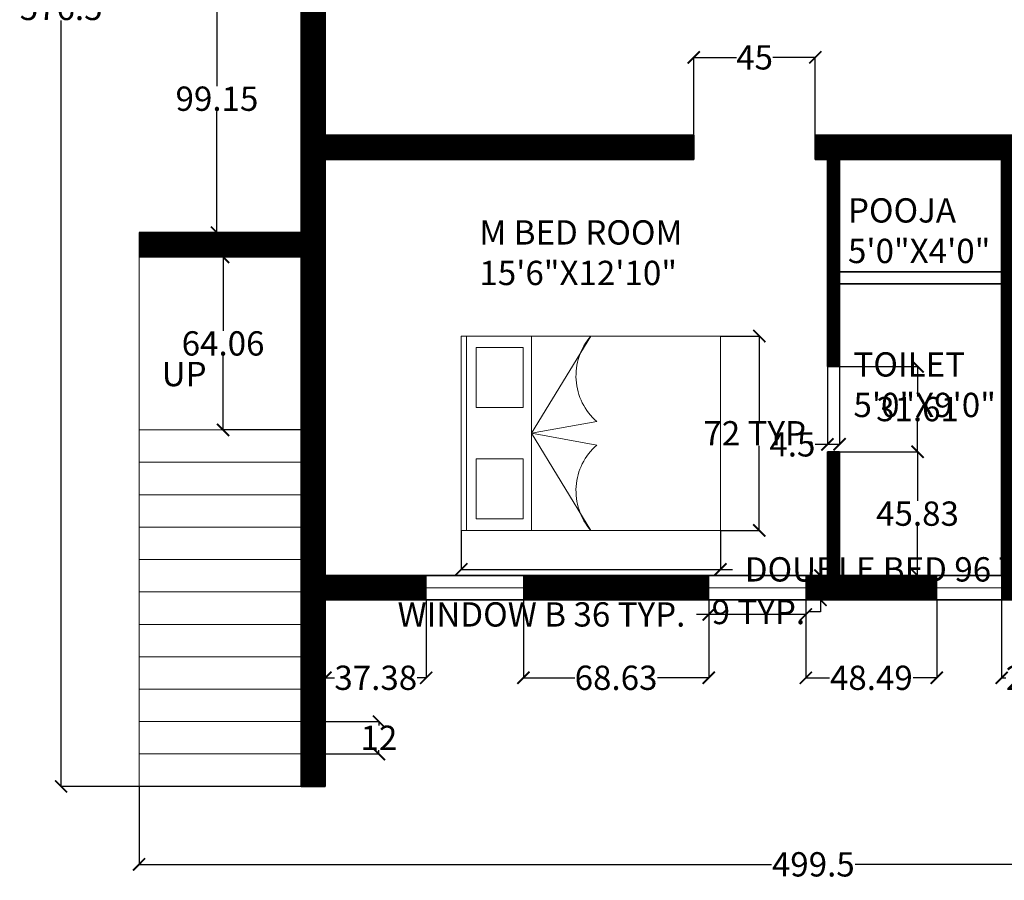
# Model space of a CAD drawing. Units: inches. Extents: x -124 to 468, y -83 to 563.
# Tile 1 of 3: x -124 to 241, y -83 to 235. Entities that reach past the tile are written whole.
import ezdxf

# ---------------------------------------------------------------- set-up
doc = ezdxf.new("R2010")
doc.units = ezdxf.units.IN
doc.header["$MEASUREMENT"] = 0
for name, color, linetype, lineweight in [('A-ANNO-DIMS', 2, 'Continuous', 18), ('A-ANNO-TEXT', 7, 'Continuous', 18), ('A-AREA-IDEN', 7, 'Continuous', 18), ('A-FLOR-STRS', 8, 'Continuous', 18)]:
    doc.layers.add(name, color=color, linetype=linetype, lineweight=lineweight)
for name, color, linetype, lineweight, true_color in [('A-FURN', 37, 'Continuous', 18, 0x7c5b46), ('A-GLAZ', 145, 'Continuous', 18, 0x2a88b7), ('A-WALL', 149, 'Continuous', 35, 0x414448), ('A-WALL-PATT', 251, 'Continuous', 13, 0x585a5e)]:
    doc.layers.add(name, color=color, linetype=linetype, lineweight=lineweight, true_color=true_color)
doc.styles.get("Standard").update_dxf_attribs({"font": 'arial.ttf'})
doc.dimstyles.get("Standard").update_dxf_attribs({"dimtxt": 9, "dimasz": 4.5, "dimexe": 0.18, "dimexo": 0.0625, "dimgap": 0.09, "dimtad": 0, "dimtih": 1, "dimtoh": 1, "dimdec": 1, "dimzin": 0, "dimdsep": 46, "dimlunit": 4, "dimtxsty": 'Standard', "dimblk": 'ARCHTICK', "dimcen": 0.09, "dimadec": 0, "dimazin": 0, "dimtfac": 1, "dimtdec": 1, "dimtofl": 0, "dimtmove": 0, "dimatfit": 3, "dimfxl": 1, "dimtolj": 1, "dimtzin": 0, "dimarcsym": 0})

# ---------------------------------------------------------------- blocks, each defined once
blk = doc.blocks.new('BED-DOUBLE')
for p, q in [((0, 0), (0, 72)), ((0, 72), (96, 72)), ((2, 0), (2, 72)), ((26, 0), (26, 72)), ((48, 72), (26, 36)), ((96, 72), (96, 0)), ((26, 36), (50.21, 40.36)), ((26, 36), (48, 0)), ((26, 36), (50.21, 31.64)), ((50.21, 31.64), (26, 36)), ((96, 0), (0, 0))]:
    blk.add_line(p, q)
for points in [[(5.47, 67.74), (5.47, 45.52), (22.92, 45.52), (22.92, 67.74)], [(5.47, 4.26), (5.47, 26.48), (22.92, 26.48), (22.92, 4.26)]]:
    blk.add_lwpolyline(points, close=True)
for centre, start, end in [((64.91, 57.28), 138.9727, 229.0026), ((64.91, 14.72), 130.9974, 221.0273)]:
    blk.add_arc(centre, 22.42, start, end)
blk = doc.blocks.new('WIN-24IN')
for p, q in [((0, 0), (0, 9)), ((24, 0), (24, 9)), ((0, 4.5), (24, 4.5))]:
    blk.add_line(p, q)
blk = doc.blocks.new('WIN-36IN')
for p, q in [((0, 9), (0, 0)), ((36, 9), (36, 0)), ((0, 4.5), (36, 4.5))]:
    blk.add_line(p, q)
blk = doc.blocks.new('_ArchTick')
at = {"color": 0, "linetype": 'ByBlock', "const_width": 0.15}
blk.add_lwpolyline([(-0.5, -0.5), (0.5, 0.5)], dxfattribs=at)
blk = doc.blocks.new('*D6')
at = {"layer": 'A-ANNO-DIMS', "color": 0, "lineweight": -2, "transparency": 16777216}
for p, q in [((39.84, 46.01), (39.84, 31.49)), ((135.84, 46.01), (135.84, 31.49)), ((39.84, 31.67), (135.84, 31.67)), ((135.84, 31.67), (140.34, 31.67))]:
    blk.add_line(p, q, dxfattribs=at)
at = {"layer": 'Defpoints', "color": 0, "transparency": 16777216}
for p in [(39.84, 46.07), (135.84, 46.07), (135.84, 31.67)]:
    blk.add_point(p, dxfattribs=at)
at = {"layer": 'A-ANNO-DIMS', "color": 0, "lineweight": -2, "transparency": 16777216, "xscale": 4.5, "yscale": 4.5, "zscale": 4.5, "rotation": 180}
blk.add_blockref('_ArchTick', (39.84, 31.67), dxfattribs=at)
at = {"layer": 'A-ANNO-DIMS', "color": 0, "lineweight": -2, "transparency": 16777216, "xscale": 4.5, "yscale": 4.5, "zscale": 4.5}
blk.add_blockref('_ArchTick', (135.84, 31.67), dxfattribs=at)
at = {"layer": 'A-ANNO-DIMS', "color": 0, "transparency": 16777216, "insert": (204.38, 31.67), "char_height": 9, "attachment_point": 5}
blk.add_mtext('\\A1;DOUBLE BED 96 TYP.', dxfattribs=at)
blk = doc.blocks.new('*D7')
at = {"layer": 'A-ANNO-DIMS', "color": 0, "lineweight": -2, "transparency": 16777216}
for p, q in [((135.9, 118.07), (150.42, 118.07)), ((150.24, 118.07), (150.24, 86.68)), ((150.24, 46.07), (150.24, 77.46)), ((135.9, 46.07), (150.42, 46.07))]:
    blk.add_line(p, q, dxfattribs=at)
at = {"layer": 'Defpoints', "color": 0, "transparency": 16777216}
for p in [(135.84, 118.07), (150.24, 118.07), (135.84, 46.07)]:
    blk.add_point(p, dxfattribs=at)
at = {"layer": 'A-ANNO-DIMS', "color": 0, "lineweight": -2, "transparency": 16777216, "xscale": 4.5, "yscale": 4.5, "zscale": 4.5}
for p, rotation in [((150.24, 118.07), 90), ((150.24, 46.07), 270)]:
    blk.add_blockref('_ArchTick', p, dxfattribs=dict(at, rotation=rotation))
at = {"layer": 'A-ANNO-DIMS', "color": 0, "transparency": 16777216, "insert": (150.24, 82.07), "char_height": 9, "attachment_point": 5}
blk.add_mtext('\\A1;72 TYP.', dxfattribs=at)
blk = doc.blocks.new('*D10')
at = {"layer": 'A-ANNO-DIMS', "color": 0, "lineweight": -2, "transparency": 16777216}
for p, q in [((131.49, 20.33), (131.49, 14.81)), ((167.49, 20.33), (167.49, 14.81)), ((131.49, 14.99), (126.99, 14.99)), ((167.49, 14.99), (131.49, 14.99))]:
    blk.add_line(p, q, dxfattribs=at)
at = {"layer": 'Defpoints', "color": 0, "transparency": 16777216}
for p in [(131.49, 20.39), (167.49, 20.39), (131.49, 14.99)]:
    blk.add_point(p, dxfattribs=at)
at = {"layer": 'A-ANNO-DIMS', "color": 0, "lineweight": -2, "transparency": 16777216, "xscale": 4.5, "yscale": 4.5, "zscale": 4.5, "rotation": 180}
blk.add_blockref('_ArchTick', (131.49, 14.99), dxfattribs=at)
at = {"layer": 'A-ANNO-DIMS', "color": 0, "lineweight": -2, "transparency": 16777216, "xscale": 4.5, "yscale": 4.5, "zscale": 4.5}
blk.add_blockref('_ArchTick', (167.49, 14.99), dxfattribs=at)
at = {"layer": 'A-ANNO-DIMS', "color": 0, "transparency": 16777216, "insert": (69.54, 14.99), "char_height": 9, "attachment_point": 5}
blk.add_mtext('\\A1;WINDOW B 36 TYP.', dxfattribs=at)
blk = doc.blocks.new('*D11')
at = {"layer": 'A-ANNO-DIMS', "color": 0, "lineweight": -2, "transparency": 16777216}
for p, q in [((167.55, 29.39), (173.07, 29.39)), ((172.89, 29.39), (172.89, 20.39)), ((167.55, 20.39), (173.07, 20.39)), ((172.89, 20.39), (172.89, 15.89)), ((172.89, 15.89), (168.39, 15.89))]:
    blk.add_line(p, q, dxfattribs=at)
at = {"layer": 'Defpoints', "color": 0, "transparency": 16777216}
for p in [(167.49, 29.39), (167.49, 20.39), (172.89, 20.39)]:
    blk.add_point(p, dxfattribs=at)
at = {"layer": 'A-ANNO-DIMS', "color": 0, "lineweight": -2, "transparency": 16777216, "xscale": 4.5, "yscale": 4.5, "zscale": 4.5}
for p, rotation in [((172.89, 29.39), 90), ((172.89, 20.39), 270)]:
    blk.add_blockref('_ArchTick', p, dxfattribs=dict(at, rotation=rotation))
at = {"layer": 'A-ANNO-DIMS', "color": 0, "transparency": 16777216, "insert": (149.89, 15.89), "char_height": 9, "attachment_point": 5}
blk.add_mtext('\\A1;9 TYP.', dxfattribs=at)
blk = doc.blocks.new('*D14')
at = {"layer": 'A-ANNO-DIMS', "color": 0, "lineweight": -2, "transparency": 16777216}
for p, q in [((419.98, 183.33), (419.98, -77.73)), ((-79.52, -48.75), (-79.52, -77.73)), ((-79.52, -77.55), (154.74, -77.55)), ((419.98, -77.55), (185.72, -77.55))]:
    blk.add_line(p, q, dxfattribs=at)
at = {"layer": 'Defpoints', "color": 0, "transparency": 16777216}
for p in [(419.98, 183.39), (-79.52, -48.69), (419.98, -77.55)]:
    blk.add_point(p, dxfattribs=at)
at = {"layer": 'A-ANNO-DIMS', "color": 0, "lineweight": -2, "transparency": 16777216, "xscale": 4.5, "yscale": 4.5, "zscale": 4.5, "rotation": 180}
blk.add_blockref('_ArchTick', (-79.52, -77.55), dxfattribs=at)
at = {"layer": 'A-ANNO-DIMS', "color": 0, "lineweight": -2, "transparency": 16777216, "xscale": 4.5, "yscale": 4.5, "zscale": 4.5}
blk.add_blockref('_ArchTick', (419.98, -77.55), dxfattribs=at)
at = {"layer": 'A-ANNO-DIMS', "color": 0, "transparency": 16777216, "insert": (170.23, -77.55), "char_height": 9, "attachment_point": 5}
blk.add_mtext('\\A1;499.5', dxfattribs=at)
blk = doc.blocks.new('*D15')
at = {"layer": 'A-ANNO-DIMS', "color": 0, "lineweight": -2, "transparency": 16777216}
for p, q in [((-19.59, 527.82), (-108.57, 527.82)), ((-108.39, 527.82), (-108.39, 244.25)), ((-108.39, -48.69), (-108.39, 234.88)), ((-19.59, -48.69), (-108.57, -48.69))]:
    blk.add_line(p, q, dxfattribs=at)
at = {"layer": 'Defpoints', "color": 0, "transparency": 16777216}
for p in [(-108.39, 527.82), (-19.52, 527.82), (-19.52, -48.69)]:
    blk.add_point(p, dxfattribs=at)
at = {"layer": 'A-ANNO-DIMS', "color": 0, "lineweight": -2, "transparency": 16777216, "xscale": 4.5, "yscale": 4.5, "zscale": 4.5}
for p, rotation in [((-108.39, 527.82), 90), ((-108.39, -48.69), 270)]:
    blk.add_blockref('_ArchTick', p, dxfattribs=dict(at, rotation=rotation))
at = {"layer": 'A-ANNO-DIMS', "color": 0, "transparency": 16777216, "insert": (-108.39, 239.57), "char_height": 9, "attachment_point": 5}
blk.add_mtext('\\A1;576.5', dxfattribs=at)
blk = doc.blocks.new('*D28')
at = {"layer": 'A-ANNO-DIMS', "color": 0, "lineweight": -2, "transparency": 16777216}
for p, q in [((-10.52, 20.33), (-10.52, -8.65)), ((26.86, 20.33), (26.86, -8.65)), ((-10.52, -8.47), (-7.11, -8.47)), ((26.86, -8.47), (23.45, -8.47))]:
    blk.add_line(p, q, dxfattribs=at)
at = {"layer": 'Defpoints', "color": 0, "transparency": 16777216}
for p in [(-10.52, 20.39), (26.86, 20.39), (-10.52, -8.47)]:
    blk.add_point(p, dxfattribs=at)
at = {"layer": 'A-ANNO-DIMS', "color": 0, "lineweight": -2, "transparency": 16777216, "xscale": 4.5, "yscale": 4.5, "zscale": 4.5, "rotation": 180}
blk.add_blockref('_ArchTick', (-10.52, -8.47), dxfattribs=at)
at = {"layer": 'A-ANNO-DIMS', "color": 0, "lineweight": -2, "transparency": 16777216, "xscale": 4.5, "yscale": 4.5, "zscale": 4.5}
blk.add_blockref('_ArchTick', (26.86, -8.47), dxfattribs=at)
at = {"layer": 'A-ANNO-DIMS', "color": 0, "transparency": 16777216, "insert": (8.17, -8.47), "char_height": 9, "attachment_point": 5}
blk.add_mtext('\\A1;37.38', dxfattribs=at)
blk = doc.blocks.new('*D29')
at = {"layer": 'A-ANNO-DIMS', "color": 0, "lineweight": -2, "transparency": 16777216}
for p, q in [((62.86, 20.33), (62.86, -8.65)), ((131.49, 20.33), (131.49, -8.65)), ((62.86, -8.47), (81.87, -8.47)), ((131.49, -8.47), (112.47, -8.47))]:
    blk.add_line(p, q, dxfattribs=at)
at = {"layer": 'Defpoints', "color": 0, "transparency": 16777216}
for p in [(62.86, 20.39), (131.49, 20.39), (62.86, -8.47)]:
    blk.add_point(p, dxfattribs=at)
at = {"layer": 'A-ANNO-DIMS', "color": 0, "lineweight": -2, "transparency": 16777216, "xscale": 4.5, "yscale": 4.5, "zscale": 4.5, "rotation": 180}
blk.add_blockref('_ArchTick', (62.86, -8.47), dxfattribs=at)
at = {"layer": 'A-ANNO-DIMS', "color": 0, "lineweight": -2, "transparency": 16777216, "xscale": 4.5, "yscale": 4.5, "zscale": 4.5}
blk.add_blockref('_ArchTick', (131.49, -8.47), dxfattribs=at)
at = {"layer": 'A-ANNO-DIMS', "color": 0, "transparency": 16777216, "insert": (97.17, -8.47), "char_height": 9, "attachment_point": 5}
blk.add_mtext('\\A1;68.63', dxfattribs=at)
blk = doc.blocks.new('*D30')
at = {"layer": 'A-ANNO-DIMS', "color": 0, "lineweight": -2, "transparency": 16777216}
for p, q in [((167.49, 20.33), (167.49, -8.65)), ((215.98, 20.33), (215.98, -8.65)), ((167.49, -8.47), (176.27, -8.47)), ((215.98, -8.47), (207.2, -8.47))]:
    blk.add_line(p, q, dxfattribs=at)
at = {"layer": 'Defpoints', "color": 0, "transparency": 16777216}
for p in [(167.49, 20.39), (215.98, 20.39), (167.49, -8.47)]:
    blk.add_point(p, dxfattribs=at)
at = {"layer": 'A-ANNO-DIMS', "color": 0, "lineweight": -2, "transparency": 16777216, "xscale": 4.5, "yscale": 4.5, "zscale": 4.5}
for p, rotation in [((167.49, -8.47), 179.9999999999999), ((215.98, -8.47), 359.9999999999999)]:
    blk.add_blockref('_ArchTick', p, dxfattribs=dict(at, rotation=rotation))
at = {"layer": 'A-ANNO-DIMS', "color": 0, "transparency": 16777216, "insert": (191.73, -8.47), "char_height": 9, "attachment_point": 5}
blk.add_mtext('\\A1;48.49', dxfattribs=at)
blk = doc.blocks.new('*D31')
at = {"layer": 'A-ANNO-DIMS', "color": 0, "lineweight": -2, "transparency": 16777216}
for p, q in [((239.98, 20.33), (239.98, -8.65)), ((266.88, 20.33), (266.88, -8.65)), ((239.98, -8.47), (241.56, -8.47)), ((266.88, -8.47), (265.29, -8.47))]:
    blk.add_line(p, q, dxfattribs=at)
at = {"layer": 'Defpoints', "color": 0, "transparency": 16777216}
for p in [(239.98, 20.39), (266.88, 20.39), (239.98, -8.47)]:
    blk.add_point(p, dxfattribs=at)
at = {"layer": 'A-ANNO-DIMS', "color": 0, "lineweight": -2, "transparency": 16777216, "xscale": 4.5, "yscale": 4.5, "zscale": 4.5, "rotation": 180.0000000000002}
blk.add_blockref('_ArchTick', (239.98, -8.47), dxfattribs=at)
at = {"layer": 'A-ANNO-DIMS', "color": 0, "lineweight": -2, "transparency": 16777216, "xscale": 4.5, "yscale": 4.5, "zscale": 4.5}
blk.add_blockref('_ArchTick', (266.88, -8.47), dxfattribs=at)
at = {"layer": 'A-ANNO-DIMS', "color": 0, "transparency": 16777216, "insert": (253.43, -8.47), "char_height": 9, "attachment_point": 5}
blk.add_mtext('\\A1;26.9', dxfattribs=at)
blk = doc.blocks.new('*D35')
at = {"layer": 'A-ANNO-DIMS', "color": 0, "lineweight": -2, "transparency": 16777216}
for p, q in [((-19.46, -24.69), (9.52, -24.69)), ((9.34, -24.69), (9.34, -26.08)), ((9.34, -36.69), (9.34, -35.3)), ((-19.46, -36.69), (9.52, -36.69))]:
    blk.add_line(p, q, dxfattribs=at)
at = {"layer": 'Defpoints', "color": 0, "transparency": 16777216}
for p in [(-19.52, -24.69), (-19.52, -36.69), (9.34, -36.69)]:
    blk.add_point(p, dxfattribs=at)
at = {"layer": 'A-ANNO-DIMS', "color": 0, "lineweight": -2, "transparency": 16777216, "xscale": 4.5, "yscale": 4.5, "zscale": 4.5}
for p, rotation in [((9.34, -24.69), 90), ((9.34, -36.69), 270)]:
    blk.add_blockref('_ArchTick', p, dxfattribs=dict(at, rotation=rotation))
at = {"layer": 'A-ANNO-DIMS', "color": 0, "transparency": 16777216, "insert": (9.34, -30.69), "char_height": 9, "attachment_point": 5}
blk.add_mtext('\\A1;12', dxfattribs=at)
blk = doc.blocks.new('*D36')
at = {"layer": 'A-ANNO-DIMS', "color": 0, "lineweight": -2, "transparency": 16777216}
for p, q in [((-79.46, 255.53), (-50.48, 255.53)), ((-50.66, 255.53), (-50.66, 210.64)), ((-50.66, 156.37), (-50.66, 201.27)), ((-79.46, 156.37), (-50.48, 156.37))]:
    blk.add_line(p, q, dxfattribs=at)
at = {"layer": 'Defpoints', "color": 0, "transparency": 16777216}
for p in [(-79.52, 255.53), (-79.52, 156.37), (-50.66, 156.37)]:
    blk.add_point(p, dxfattribs=at)
at = {"layer": 'A-ANNO-DIMS', "color": 0, "lineweight": -2, "transparency": 16777216, "xscale": 4.5, "yscale": 4.5, "zscale": 4.5}
for p, rotation in [((-50.66, 255.53), 90), ((-50.66, 156.37), 270)]:
    blk.add_blockref('_ArchTick', p, dxfattribs=dict(at, rotation=rotation))
at = {"layer": 'A-ANNO-DIMS', "color": 0, "transparency": 16777216, "insert": (-50.66, 205.95), "char_height": 9, "attachment_point": 5}
blk.add_mtext('\\A1;99.15', dxfattribs=at)
blk = doc.blocks.new('*D37')
at = {"layer": 'A-ANNO-DIMS', "color": 0, "lineweight": -2, "transparency": 16777216}
for p, q in [((-19.59, 147.37), (-48.57, 147.37)), ((-48.39, 147.37), (-48.39, 120.03)), ((-48.39, 83.31), (-48.39, 110.66)), ((-19.59, 83.31), (-48.57, 83.31))]:
    blk.add_line(p, q, dxfattribs=at)
at = {"layer": 'Defpoints', "color": 0, "transparency": 16777216}
for p in [(-48.39, 147.37), (-19.52, 147.37), (-19.52, 83.31)]:
    blk.add_point(p, dxfattribs=at)
at = {"layer": 'A-ANNO-DIMS', "color": 0, "lineweight": -2, "transparency": 16777216, "xscale": 4.5, "yscale": 4.5, "zscale": 4.5}
for p, rotation in [((-48.39, 147.37), 90), ((-48.39, 83.31), 270)]:
    blk.add_blockref('_ArchTick', p, dxfattribs=dict(at, rotation=rotation))
at = {"layer": 'A-ANNO-DIMS', "color": 0, "transparency": 16777216, "insert": (-48.39, 115.34), "char_height": 9, "attachment_point": 5}
blk.add_mtext('\\A1;64.06', dxfattribs=at)
blk = doc.blocks.new('*D40')
at = {"layer": 'A-ANNO-DIMS', "color": 0, "lineweight": -2, "transparency": 16777216}
for p, q in [((125.98, 192.46), (125.98, 221.44)), ((125.98, 221.26), (141.73, 221.26)), ((170.98, 221.26), (155.23, 221.26)), ((170.98, 192.46), (170.98, 221.44))]:
    blk.add_line(p, q, dxfattribs=at)
at = {"layer": 'Defpoints', "color": 0, "transparency": 16777216}
for p in [(170.98, 221.26), (125.98, 192.39), (170.98, 192.39)]:
    blk.add_point(p, dxfattribs=at)
at = {"layer": 'A-ANNO-DIMS', "color": 0, "lineweight": -2, "transparency": 16777216, "xscale": 4.5, "yscale": 4.5, "zscale": 4.5, "rotation": 180}
blk.add_blockref('_ArchTick', (125.98, 221.26), dxfattribs=at)
at = {"layer": 'A-ANNO-DIMS', "color": 0, "lineweight": -2, "transparency": 16777216, "xscale": 4.5, "yscale": 4.5, "zscale": 4.5}
blk.add_blockref('_ArchTick', (170.98, 221.26), dxfattribs=at)
at = {"layer": 'A-ANNO-DIMS', "color": 0, "transparency": 16777216, "insert": (148.48, 221.26), "char_height": 9, "attachment_point": 5}
blk.add_mtext('\\A1;45', dxfattribs=at)
blk = doc.blocks.new('*D41')
at = {"layer": 'A-ANNO-DIMS', "color": 0, "lineweight": -2, "transparency": 16777216}
for p, q in [((180.04, 106.83), (209.02, 106.83)), ((208.84, 106.83), (208.84, 95.72)), ((208.84, 75.22), (208.84, 86.34)), ((180.04, 75.22), (209.02, 75.22))]:
    blk.add_line(p, q, dxfattribs=at)
at = {"layer": 'Defpoints', "color": 0, "transparency": 16777216}
for p in [(179.98, 106.83), (179.98, 75.22), (208.84, 75.22)]:
    blk.add_point(p, dxfattribs=at)
at = {"layer": 'A-ANNO-DIMS', "color": 0, "lineweight": -2, "transparency": 16777216, "xscale": 4.5, "yscale": 4.5, "zscale": 4.5}
for p, rotation in [((208.84, 106.83), 90), ((208.84, 75.22), 270)]:
    blk.add_blockref('_ArchTick', p, dxfattribs=dict(at, rotation=rotation))
at = {"layer": 'A-ANNO-DIMS', "color": 0, "transparency": 16777216, "insert": (208.84, 91.03), "char_height": 9, "attachment_point": 5}
blk.add_mtext('\\A1;31.61', dxfattribs=at)
blk = doc.blocks.new('*D45')
at = {"layer": 'A-ANNO-DIMS', "color": 0, "lineweight": -2, "transparency": 16777216}
for p, q in [((180.04, 75.22), (209.02, 75.22)), ((208.84, 75.22), (208.84, 57)), ((208.84, 29.39), (208.84, 47.62)), ((180.04, 29.39), (209.02, 29.39))]:
    blk.add_line(p, q, dxfattribs=at)
at = {"layer": 'Defpoints', "color": 0, "transparency": 16777216}
for p in [(179.98, 75.22), (179.98, 29.39), (208.84, 29.39)]:
    blk.add_point(p, dxfattribs=at)
at = {"layer": 'A-ANNO-DIMS', "color": 0, "lineweight": -2, "transparency": 16777216, "xscale": 4.5, "yscale": 4.5, "zscale": 4.5}
for p, rotation in [((208.84, 75.22), 90), ((208.84, 29.39), 270)]:
    blk.add_blockref('_ArchTick', p, dxfattribs=dict(at, rotation=rotation))
at = {"layer": 'A-ANNO-DIMS', "color": 0, "transparency": 16777216, "insert": (208.84, 52.31), "char_height": 9, "attachment_point": 5}
blk.add_mtext('\\A1;45.83', dxfattribs=at)
blk = doc.blocks.new('*D46')
at = {"layer": 'A-ANNO-DIMS', "color": 0, "lineweight": -2, "transparency": 16777216}
for p, q in [((175.48, 106.77), (175.48, 77.79)), ((179.98, 106.77), (179.98, 77.79)), ((175.48, 77.97), (170.98, 77.97)), ((179.98, 77.97), (175.48, 77.97))]:
    blk.add_line(p, q, dxfattribs=at)
at = {"layer": 'Defpoints', "color": 0, "transparency": 16777216}
for p in [(175.48, 106.83), (179.98, 106.83), (175.48, 77.97)]:
    blk.add_point(p, dxfattribs=at)
at = {"layer": 'A-ANNO-DIMS', "color": 0, "lineweight": -2, "transparency": 16777216, "xscale": 4.5, "yscale": 4.5, "zscale": 4.5, "rotation": 180}
blk.add_blockref('_ArchTick', (175.48, 77.97), dxfattribs=at)
at = {"layer": 'A-ANNO-DIMS', "color": 0, "lineweight": -2, "transparency": 16777216, "xscale": 4.5, "yscale": 4.5, "zscale": 4.5}
blk.add_blockref('_ArchTick', (179.98, 77.97), dxfattribs=at)
at = {"layer": 'A-ANNO-DIMS', "color": 0, "transparency": 16777216, "insert": (162.48, 77.97), "char_height": 9, "attachment_point": 5}
blk.add_mtext('\\A1;4.5', dxfattribs=at)

msp = doc.modelspace()

# ---------------------------------------------------------------- hatches: boundary and pattern name
at = {"layer": 'A-WALL-PATT'}
h = msp.add_hatch(dxfattribs=at)
h.set_pattern_fill('ANSI31', color=256)
h.set_pattern_definition([(45, (-392.07623, 0), (-0.088388348, 0.088388348), [])])
h.paths.add_polyline_path([(377.9763, 141.7862), (377.9763, 183.3929), (419.9763, 183.3929), (419.9763, 192.3929), (419.9763, 324.3929), (419.9763, 333.3929), (377.9763, 333.3929), (377.9763, 361.0673), (368.9763, 361.0673), (368.9763, 333.3929), (290.9763, 333.3929), (290.9763, 324.3929), (323.9763, 324.3929), (323.9763, 192.3929), (323.9763, 183.3929), (368.9763, 183.3929), (368.9763, 141.7862), (368.9763, 29.3929), (343.3064, 29.3929), (343.3064, 20.3929), (377.9763, 20.3929)])
h.paths.add_polyline_path([(368.9763, 192.3929), (332.9763, 192.3929), (332.9763, 324.3929), (368.9763, 324.3929), (410.9763, 324.3929), (410.9763, 192.3929)], flags=16)
h.paths.add_polyline_path([(215.9763, 29.3929), (179.9763, 29.3929), (179.9763, 75.2245), (175.4763, 75.2245), (175.4763, 29.3929), (167.489, 29.3929), (167.489, 20.3929), (215.9763, 20.3929)])
h.paths.add_polyline_path([(266.8777, 29.3929), (244.4763, 29.3929), (244.4763, 141.7862), (244.4763, 183.3929), (257.421, 183.3929), (257.421, 192.3929), (170.9763, 192.3929), (170.9763, 183.3929), (175.4763, 183.3929), (175.4763, 141.7862), (175.4763, 106.8322), (179.9763, 106.8322), (179.9763, 141.7862), (179.9763, 183.3929), (239.9763, 183.3929), (239.9763, 141.7862), (239.9763, 29.3929), (239.9763, 20.3929), (266.8777, 20.3929)])
h.paths.add_polyline_path([(131.489, 29.3929), (62.8565, 29.3929), (62.8565, 20.3929), (131.489, 20.3929)])
h.paths.add_polyline_path([(26.8565, 29.3929), (-10.5237, 29.3929), (-10.5237, 141.7862), (-10.5237, 183.3929), (125.9763, 183.3929), (125.9763, 192.3929), (-10.5237, 192.3929), (-10.5237, 324.3929), (125.9763, 324.3929), (125.9763, 333.3929), (-10.5237, 333.3929), (-10.5237, 477.3929), (23.4837, 477.3929), (23.4837, 486.3929), (-10.5237, 486.3929), (-10.5237, 527.8228), (-19.5237, 527.8228), (-19.5237, 486.3929), (-19.5237, 264.528), (-79.5237, 264.528), (-79.5237, 255.528), (-19.5237, 255.528), (-19.5237, 156.3747), (-79.5237, 156.3747), (-79.5237, 147.3747), (-19.5237, 147.3747), (-19.5237, 141.7862), (-19.5237, -48.6869), (-10.5237, -48.6869), (-10.5237, 20.3929), (26.8565, 20.3929)])
h.paths.add_polyline_path([(220.4763, 486.3929), (149.9763, 486.3929), (149.9763, 477.3929), (185.9763, 477.3929), (185.9763, 381.3929), (125.9763, 381.3929), (125.9763, 428.759), (121.4763, 428.759), (121.4763, 376.8929), (125.9763, 376.8929), (185.9763, 376.8929), (185.9763, 333.3929), (174.9252, 333.3929), (174.9252, 324.3929), (190.4763, 324.3929), (190.4763, 333.3929), (190.4763, 349.8929), (244.4763, 349.8929), (244.4763, 333.3929), (244.4763, 324.3929), (248.9763, 324.3929), (248.9763, 333.3929), (248.9763, 428.759), (244.4763, 428.759), (244.4763, 354.3929), (190.4763, 354.3929), (190.4763, 477.3929), (220.4763, 477.3929)])
h.paths.add_polyline_path([(377.9763, 486.3929), (310.948, 486.3929), (310.948, 477.3929), (368.9763, 477.3929), (368.9763, 385.0673), (377.9763, 385.0673)])
h.paths.add_polyline_path([(339.1974, 237.2234), (400.8652, 237.2234), (400.8652, 270.8067), (339.1974, 270.8067)], flags=8)
h.paths.add_polyline_path([(182.8614, 357.8948), (247.9303, 357.8948), (247.9303, 391.478), (182.8614, 391.478)], flags=25)

# ---------------------------------------------------------------- linework, layer by layer
at = {"layer": 'A-FLOR-STRS'}
for p, q in [((-79.5237, 156.3747), (-79.5237, 141.7862)), ((-79.5237, 141.7862), (-79.5237, -48.6869)), ((-79.5237, 83.3131), (-19.5237, 83.3131)), ((-79.5237, 71.3131), (-19.5237, 71.3131)), ((-79.5237, 59.3131), (-19.5237, 59.3131)), ((-79.5237, 47.3131), (-19.5237, 47.3131)), ((-79.5237, 35.3131), (-19.5237, 35.3131)), ((-79.5237, 23.3131), (-19.5237, 23.3131)), ((-79.5237, 11.3131), (-19.5237, 11.3131)), ((-79.5237, -0.6869), (-19.5237, -0.6869)), ((-79.5237, -12.6869), (-19.5237, -12.6869)), ((-79.5237, -24.6869), (-19.5237, -24.6869)), ((-79.5237, -36.6869), (-19.5237, -36.6869)), ((-79.5237, -48.6869), (-19.5237, -48.6869))]:
    msp.add_line(p, q, dxfattribs=at)
at = {"layer": 'A-WALL'}
for p, q in [((-10.5237, 324.3929), (-10.5237, 192.3929)), ((-19.5237, 255.528), (-19.5237, 156.3747)), ((-10.5237, 192.3929), (125.9763, 192.3929)), ((125.9763, 192.3929), (125.9763, 183.3929)), ((170.9763, 183.3929), (170.9763, 192.3929)), ((170.9763, 192.3929), (257.421, 192.3929)), ((-10.5237, 183.3929), (125.9763, 183.3929)), ((-10.5237, 183.3929), (-10.5237, 141.7862)), ((170.9763, 183.3929), (175.4763, 183.3929)), ((175.4763, 183.3929), (175.4763, 141.7862)), ((179.9763, 183.3929), (179.9763, 141.7862)), ((179.9763, 183.3929), (239.9763, 183.3929)), ((239.9763, 183.3929), (239.9763, 141.7862)), ((-79.5237, 156.3747), (-19.5237, 156.3747)), ((-79.5237, 147.3747), (-19.5237, 147.3747)), ((-19.5237, 147.3747), (-19.5237, 141.7862)), ((-19.5237, 141.7862), (-19.5237, -48.6869)), ((-10.5237, 141.7862), (-10.5237, 29.3929)), ((175.4763, 141.7862), (175.4763, 106.8322)), ((179.9763, 141.8929), (239.9763, 141.8929)), ((179.9763, 141.7862), (179.9763, 106.8322)), ((239.9763, 141.7862), (239.9763, 29.3929)), ((179.9763, 137.3929), (239.9763, 137.3929)), ((175.4763, 106.8322), (179.9763, 106.8322)), ((175.4763, 75.2245), (179.9763, 75.2245)), ((175.4763, 75.2245), (175.4763, 29.3929)), ((179.9763, 75.2245), (179.9763, 29.3929)), ((-10.5237, 29.3929), (175.4763, 29.3929)), ((179.9763, 29.3929), (239.9763, 29.3929)), ((-10.5237, 20.3929), (377.9763, 20.3929)), ((-10.5237, 20.3929), (-10.5237, -48.6869)), ((-19.5237, -48.6869), (-10.5237, -48.6869))]:
    msp.add_line(p, q, dxfattribs=at)

# ---------------------------------------------------------------- block references
at = {"layer": 'A-FURN'}
msp.add_blockref('BED-DOUBLE', (39.8352, 46.0706), dxfattribs=at)
at = {"layer": 'A-GLAZ'}
msp.add_blockref('WIN-36IN', (26.856, 20.393), dxfattribs=at)
at = {"layer": 'A-GLAZ', "rotation": 180}
for name, p in [('WIN-36IN', (167.4895, 29.3927)), ('WIN-24IN', (239.9766, 29.3927))]:
    msp.add_blockref(name, p, dxfattribs=at)

# ---------------------------------------------------------------- texts
at = {"layer": 'A-ANNO-TEXT', "insert": (-71.1259, 108.4941), "char_height": 9, "attachment_point": 1}
msp.add_mtext_dynamic_manual_height_columns('UP', width=177.374172, gutter_width=1, heights=[0], dxfattribs=at)
at = {"layer": 'A-AREA-IDEN', "char_height": 9, "attachment_point": 1}
for s, insert in [('POOJA\\P5\'0"X4\'0"', (183.0737, 169.0844)), ('M BED ROOM\\P15\'6"X12\'10"', (46.5497, 160.9378)), ('TOILET\\P5\'0"X9\'0"', (185.1114, 112.0583))]:
    msp.add_mtext_dynamic_manual_height_columns(s, width=177.374172, gutter_width=1, heights=[0], dxfattribs=dict(at, insert=insert))

# ---------------------------------------------------------------- dimensions: what is measured, and where the dimension line sits
at = {"layer": 'A-ANNO-DIMS'}
for base, p1, p2, angle, override, picture, middle in [((-108.3887, 527.8228), (-19.5237, -48.6869), (-19.5237, 527.8228), 90, {"dimdec": 1, "dimlfac": 1, "dimrnd": 0, "dimzin": 0, "dimdsep": 46, "dimlunit": 2}, '*D15', (-108.3887, 239.5679)), ((-50.6587, 156.3747), (-79.5237, 255.528), (-79.5237, 156.3747), 270, {"dimdec": 2, "dimlfac": 1, "dimrnd": 0, "dimzin": 0, "dimdsep": 46, "dimlunit": 2}, '*D36', (-50.6587, 205.9513)), ((-48.3887, 147.3747), (-19.5237, 83.3131), (-19.5237, 147.3747), 90, {"dimdec": 2, "dimlfac": 1, "dimrnd": 0, "dimzin": 0, "dimdsep": 46, "dimlunit": 2}, '*D37', (-48.3887, 115.3439)), ((175.4763, 77.9672), (179.9763, 106.8322), (175.4763, 106.8322), 180, {"dimdec": 1, "dimlfac": 1, "dimrnd": 0, "dimzin": 0, "dimdsep": 46, "dimlunit": 2}, '*D46', (162.4787, 77.9672)), ((208.8413, 75.2245), (179.9763, 106.8322), (179.9763, 75.2245), 270, {"dimdec": 2, "dimlfac": 1, "dimrnd": 0, "dimzin": 0, "dimdsep": 46, "dimlunit": 2}, '*D41', (208.8413, 91.0283)), ((208.8413, 29.3929), (179.9763, 75.2245), (179.9763, 29.3929), 270, {"dimdec": 2, "dimlfac": 1, "dimrnd": 0, "dimzin": 0, "dimdsep": 46, "dimlunit": 2}, '*D45', (208.8413, 52.3087)), ((-10.5237, -8.4721), (26.8565, 20.3929), (-10.5237, 20.3929), 180, {"dimdec": 2, "dimlfac": 1, "dimrnd": 0, "dimzin": 0, "dimdsep": 46, "dimlunit": 2}, '*D28', (8.1664, -8.4721)), ((62.8565, -8.4721), (131.489, 20.3929), (62.8565, 20.3929), 180, {"dimdec": 2, "dimlfac": 1, "dimrnd": 0, "dimzin": 0, "dimdsep": 46, "dimlunit": 2}, '*D29', (97.1727, -8.4721)), ((167.489, -8.4721), (215.9763, 20.3929), (167.489, 20.3929), 180, {"dimdec": 2, "dimlfac": 1, "dimrnd": 0, "dimzin": 0, "dimdsep": 46, "dimlunit": 2}, '*D30', (191.7326, -8.4721)), ((239.9763, -8.4721), (266.8777, 20.3929), (239.9763, 20.3929), 180, {"dimdec": 1, "dimlfac": 1, "dimrnd": 0, "dimzin": 0, "dimdsep": 46, "dimlunit": 2}, '*D31', (253.427, -8.4721)), ((9.3413, -36.6869), (-19.5237, -24.6869), (-19.5237, -36.6869), 270, {"dimdec": 0, "dimlfac": 1, "dimrnd": 0, "dimzin": 0, "dimdsep": 46, "dimlunit": 2}, '*D35', (9.3413, -30.6869))]:
    dim = msp.add_linear_dim(base=base, p1=p1, p2=p2, angle=angle, dimstyle='Standard', override=override, dxfattribs=at)
    dim.commit()
    dim.dimension.update_dxf_attribs({"geometry": picture, "text_midpoint": middle})
for base, p1, p2, override, picture, middle in [((170.9763, 221.2579), (125.9763, 192.3929), (170.9763, 192.3929), {"dimdec": 0, "dimlfac": 1, "dimrnd": 0, "dimzin": 0, "dimdsep": 46, "dimlunit": 2}, '*D40', (148.4763, 221.2579)), ((419.9763, -77.5519), (-79.5237, -48.6869), (419.9763, 183.3929), {"dimdec": 1, "dimlfac": 1, "dimrnd": 0, "dimzin": 0, "dimdsep": 46, "dimlunit": 2}, '*D14', (170.2263, -77.5519))]:
    dim = msp.add_linear_dim(base=base, p1=p1, p2=p2, dimstyle='Standard', override=override, dxfattribs=at)
    dim.commit()
    dim.dimension.update_dxf_attribs({"geometry": picture, "text_midpoint": middle})
for base, p1, p2, angle, text, picture, middle in [((150.2352, 118.0703), (135.8352, 46.0703), (135.8352, 118.0703), 90, '<> TYP.', '*D7', (150.2352, 82.0703)), ((131.489, 14.9929), (167.489, 20.3929), (131.489, 20.3929), 180, 'WINDOW B <> TYP.', '*D10', (69.5409, 14.9929)), ((172.889, 20.3929), (167.489, 29.3929), (167.489, 20.3929), 270, '<> TYP.', '*D11', (149.8907, 15.8929))]:
    dim = msp.add_linear_dim(base=base, p1=p1, p2=p2, angle=angle, text=text, dimstyle='Standard', override={"dimdec": 0, "dimlfac": 1, "dimrnd": 0, "dimzin": 0, "dimdsep": 46, "dimlunit": 2}, dxfattribs=at)
    dim.commit()
    dim.dimension.update_dxf_attribs({"geometry": picture, "text_midpoint": middle})
dim = msp.add_linear_dim(base=(135.8352, 31.6703), p1=(39.8352, 46.0703), p2=(135.8352, 46.0703), text='DOUBLE BED <> TYP.', dimstyle='Standard', override={"dimdec": 0, "dimlfac": 1, "dimrnd": 0, "dimzin": 0, "dimdsep": 46, "dimlunit": 2}, dxfattribs=at)
dim.commit()
dim.dimension.update_dxf_attribs({"geometry": '*D6', "text_midpoint": (204.3768, 31.6703)})

doc.saveas('drawing.dxf')
